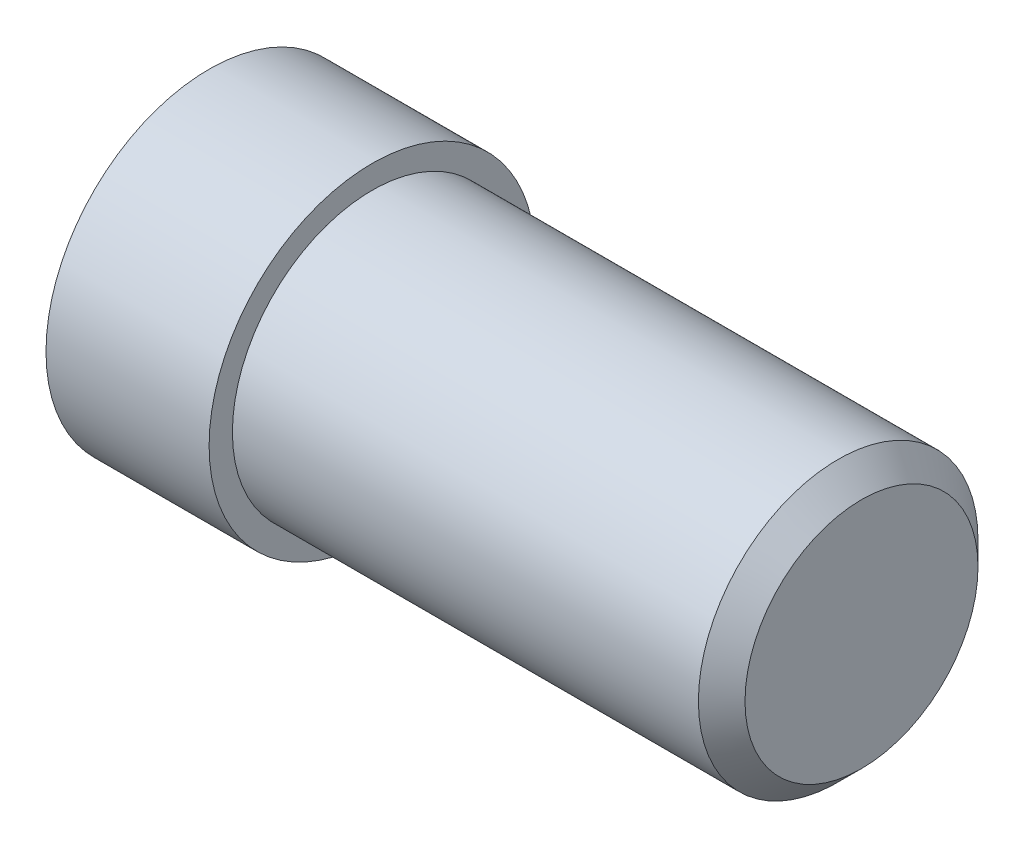
ISO-10303-21;
HEADER;
FILE_DESCRIPTION(('STEP AP214'),'2;1');
FILE_NAME('part.step','',(''),(''),'','','');
FILE_SCHEMA(('AUTOMOTIVE_DESIGN { 1 0 10303 214 1 1 1 1 }'));
ENDSEC;
DATA;
#1=APPLICATION_CONTEXT('core data for automotive mechanical design processes');
#2=APPLICATION_PROTOCOL_DEFINITION('international standard','automotive_design',2000,#1);
#3=PRODUCT_CONTEXT('',#1,'mechanical');
#4=PRODUCT('Part','Part','',(#3));
#5=PRODUCT_RELATED_PRODUCT_CATEGORY('part','',(#4));
#6=PRODUCT_DEFINITION_FORMATION('','',#4);
#7=PRODUCT_DEFINITION_CONTEXT('part definition',#1,'design');
#8=PRODUCT_DEFINITION('design','',#6,#7);
#9=PRODUCT_DEFINITION_SHAPE('','',#8);
#10=(LENGTH_UNIT() NAMED_UNIT(*) SI_UNIT(.MILLI.,.METRE.));
#11=(NAMED_UNIT(*) PLANE_ANGLE_UNIT() SI_UNIT($,.RADIAN.));
#12=(NAMED_UNIT(*) SI_UNIT($,.STERADIAN.) SOLID_ANGLE_UNIT());
#13=UNCERTAINTY_MEASURE_WITH_UNIT(LENGTH_MEASURE(1.E-05),#10,'distance_accuracy_value','');
#14=(GEOMETRIC_REPRESENTATION_CONTEXT(3) GLOBAL_UNCERTAINTY_ASSIGNED_CONTEXT((#13)) GLOBAL_UNIT_ASSIGNED_CONTEXT((#10,
#11,#12)) REPRESENTATION_CONTEXT('',''));
#15=CARTESIAN_POINT('',(0.,0.,0.));
#16=DIRECTION('',(0.,0.,1.));
#17=DIRECTION('',(1.,0.,0.));
#18=AXIS2_PLACEMENT_3D('',#15,#16,#17);
#19=CARTESIAN_POINT('',(-7.,7.,0.));
#20=DIRECTION('',(1.,0.,0.));
#21=DIRECTION('',(0.,0.,-1.));
#22=AXIS2_PLACEMENT_3D('',#19,#20,#21);
#23=PLANE('',#22);
#24=CARTESIAN_POINT('',(-7.,0.,0.));
#25=DIRECTION('',(-1.,0.,0.));
#26=DIRECTION('',(0.,0.,1.));
#27=AXIS2_PLACEMENT_3D('',#24,#25,#26);
#28=CIRCLE('',#27,7.);
#29=CARTESIAN_POINT('',(-7.,0.,7.));
#30=VERTEX_POINT('',#29);
#31=EDGE_CURVE('E65',#30,#30,#28,.T.);
#32=ORIENTED_EDGE('',*,*,#31,.T.);
#33=EDGE_LOOP('',(#32));
#34=FACE_BOUND('',#33,.T.);
#35=ADVANCED_FACE('F41',(#34),#23,.F.);
#36=CARTESIAN_POINT('',(21.,0.,0.));
#37=DIRECTION('',(-1.,0.,0.));
#38=DIRECTION('',(0.,0.,1.));
#39=AXIS2_PLACEMENT_3D('',#36,#37,#38);
#40=PLANE('',#39);
#41=CARTESIAN_POINT('',(21.,0.,0.));
#42=DIRECTION('',(-1.,0.,0.));
#43=DIRECTION('',(0.,0.,1.));
#44=AXIS2_PLACEMENT_3D('',#41,#42,#43);
#45=CIRCLE('',#44,4.99999999999999);
#46=CARTESIAN_POINT('',(21.,0.,4.99999999999999));
#47=VERTEX_POINT('',#46);
#48=EDGE_CURVE('E10',#47,#47,#45,.F.);
#49=ORIENTED_EDGE('',*,*,#48,.T.);
#50=EDGE_LOOP('',(#49));
#51=FACE_BOUND('',#50,.T.);
#52=ADVANCED_FACE('F83',(#51),#40,.F.);
#53=CARTESIAN_POINT('',(0.,0.,0.));
#54=DIRECTION('',(-1.,0.,0.));
#55=DIRECTION('',(0.,0.,1.));
#56=AXIS2_PLACEMENT_3D('',#53,#54,#55);
#57=CYLINDRICAL_SURFACE('',#56,6.);
#58=CARTESIAN_POINT('',(20.,0.,0.));
#59=DIRECTION('',(-1.,0.,0.));
#60=DIRECTION('',(0.,0.,1.));
#61=AXIS2_PLACEMENT_3D('',#58,#59,#60);
#62=CIRCLE('',#61,6.);
#63=CARTESIAN_POINT('',(20.,0.,6.));
#64=VERTEX_POINT('',#63);
#65=EDGE_CURVE('E47',#64,#64,#62,.T.);
#66=ORIENTED_EDGE('',*,*,#65,.T.);
#67=EDGE_LOOP('',(#66));
#68=FACE_BOUND('',#67,.T.);
#69=CARTESIAN_POINT('',(0.,0.,0.));
#70=DIRECTION('',(-1.,0.,0.));
#71=DIRECTION('',(0.,0.,1.));
#72=AXIS2_PLACEMENT_3D('',#69,#70,#71);
#73=CIRCLE('',#72,6.);
#74=CARTESIAN_POINT('',(0.,0.,6.));
#75=VERTEX_POINT('',#74);
#76=EDGE_CURVE('E52',#75,#75,#73,.T.);
#77=ORIENTED_EDGE('',*,*,#76,.F.);
#78=EDGE_LOOP('',(#77));
#79=FACE_BOUND('',#78,.T.);
#80=ADVANCED_FACE('F76',(#68,#79),#57,.T.);
#81=CARTESIAN_POINT('',(0.,6.,0.));
#82=DIRECTION('',(-1.,0.,0.));
#83=DIRECTION('',(0.,0.,1.));
#84=AXIS2_PLACEMENT_3D('',#81,#82,#83);
#85=PLANE('',#84);
#86=CARTESIAN_POINT('',(0.,0.,0.));
#87=DIRECTION('',(-1.,0.,0.));
#88=DIRECTION('',(0.,0.,1.));
#89=AXIS2_PLACEMENT_3D('',#86,#87,#88);
#90=CIRCLE('',#89,7.);
#91=CARTESIAN_POINT('',(0.,0.,7.));
#92=VERTEX_POINT('',#91);
#93=EDGE_CURVE('E60',#92,#92,#90,.T.);
#94=ORIENTED_EDGE('',*,*,#93,.F.);
#95=EDGE_LOOP('',(#94));
#96=FACE_BOUND('',#95,.T.);
#97=ORIENTED_EDGE('',*,*,#76,.T.);
#98=EDGE_LOOP('',(#97));
#99=FACE_BOUND('',#98,.T.);
#100=ADVANCED_FACE('F69',(#96,#99),#85,.F.);
#101=CARTESIAN_POINT('',(0.,0.,0.));
#102=DIRECTION('',(-1.,0.,0.));
#103=DIRECTION('',(0.,0.,1.));
#104=AXIS2_PLACEMENT_3D('',#101,#102,#103);
#105=CYLINDRICAL_SURFACE('',#104,7.);
#106=ORIENTED_EDGE('',*,*,#31,.F.);
#107=EDGE_LOOP('',(#106));
#108=FACE_BOUND('',#107,.T.);
#109=ORIENTED_EDGE('',*,*,#93,.T.);
#110=EDGE_LOOP('',(#109));
#111=FACE_BOUND('',#110,.T.);
#112=ADVANCED_FACE('F70',(#108,#111),#105,.T.);
#113=CARTESIAN_POINT('',(20.,0.,0.));
#114=DIRECTION('',(-1.,0.,0.));
#115=DIRECTION('',(0.,0.,1.));
#116=AXIS2_PLACEMENT_3D('',#113,#114,#115);
#117=CONICAL_SURFACE('',#116,6.,0.78539816339745);
#118=ORIENTED_EDGE('',*,*,#48,.F.);
#119=EDGE_LOOP('',(#118));
#120=FACE_BOUND('',#119,.T.);
#121=ORIENTED_EDGE('',*,*,#65,.F.);
#122=EDGE_LOOP('',(#121));
#123=FACE_BOUND('',#122,.T.);
#124=ADVANCED_FACE('F42',(#120,#123),#117,.T.);
#125=CLOSED_SHELL('',(#35,#52,#80,#100,#112,#124));
#126=MANIFOLD_SOLID_BREP('B2',#125);
#127=ADVANCED_BREP_SHAPE_REPRESENTATION('',(#18,#126),#14);
#128=SHAPE_DEFINITION_REPRESENTATION(#9,#127);
ENDSEC;
END-ISO-10303-21;
